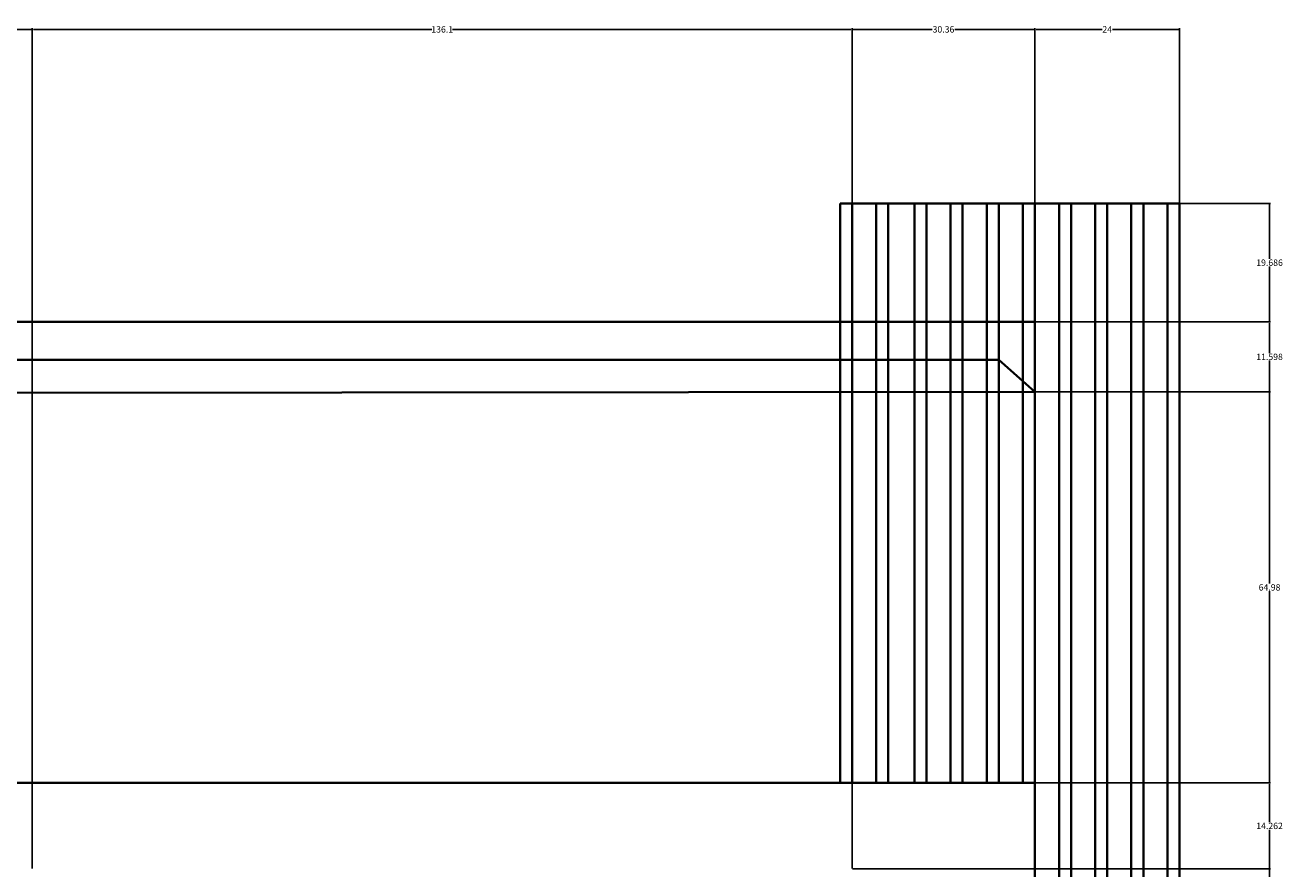
# Model space of a CAD drawing. Units: inches. Extents: x 35 to 365, y 67 to 380.
# Tile 5 of 5: x 156 to 365, y 240 to 380. Entities that reach past the tile are written whole.
import ezdxf

# ---------------------------------------------------------------- set-up
doc = ezdxf.new("R2010")
doc.units = ezdxf.units.IN
doc.header["$MEASUREMENT"] = 0
doc.layers.add('A-ANNO-DIMS', color=2, linetype='Continuous', lineweight=18)
doc.layers.add('A-FURN', color=7, linetype='Continuous', lineweight=35)
doc.styles.get("Standard").update_dxf_attribs({"font": 'arial.ttf'})
doc.dimstyles.get("Standard").update_dxf_attribs({"dimtxt": 1.0625, "dimasz": 0.18, "dimexe": 0.18, "dimexo": 0.0625, "dimgap": 0.09, "dimtad": 0, "dimtih": 1, "dimtoh": 1, "dimdec": 4, "dimzin": 0, "dimdsep": 46, "dimlunit": 4, "dimtxsty": 'Standard', "dimcen": 0.09, "dimadec": 0, "dimazin": 0, "dimtfac": 1, "dimtdec": 4, "dimtofl": 0, "dimtmove": 0, "dimatfit": 3, "dimfxl": 1, "dimtolj": 1, "dimtzin": 0, "dimarcsym": 0})

# ---------------------------------------------------------------- blocks, each defined once
blk = doc.blocks.new('*D12')
at = {"layer": 'A-ANNO-DIMS', "color": 0, "lineweight": -2, "transparency": 16777216}
for p, q in [((115.27, 351.36), (115.27, 379.42)), ((115.45, 379.24), (134.33, 379.24)), ((157.01, 379.24), (138.13, 379.24)), ((157.19, 239.87), (157.19, 379.42))]:
    blk.add_line(p, q, dxfattribs=at)
at = {"layer": 'A-ANNO-DIMS', "color": 0, "transparency": 16777216}
for points in [[(115.45, 379.27), (115.45, 379.21), (115.27, 379.24)], [(157.01, 379.27), (157.01, 379.21), (157.19, 379.24)]]:
    blk.add_solid(points, dxfattribs=at)
at = {"layer": 'Defpoints', "color": 0, "transparency": 16777216}
for p in [(157.19, 379.24), (115.27, 351.3), (157.19, 239.81)]:
    blk.add_point(p, dxfattribs=at)
at = {"layer": 'A-ANNO-DIMS', "color": 0, "transparency": 16777216, "insert": (136.23, 379.24), "char_height": 1.062, "attachment_point": 5}
blk.add_mtext('\\A1;41.92', dxfattribs=at)
blk = doc.blocks.new('*D13')
at = {"layer": 'A-ANNO-DIMS', "color": 0, "lineweight": -2, "transparency": 16777216}
for p, q in [((157.19, 239.87), (157.19, 379.42)), ((157.37, 379.24), (223.52, 379.24)), ((293.12, 379.24), (226.98, 379.24)), ((293.3, 239.87), (293.3, 379.42))]:
    blk.add_line(p, q, dxfattribs=at)
at = {"layer": 'A-ANNO-DIMS', "color": 0, "transparency": 16777216}
for points in [[(157.37, 379.27), (157.37, 379.21), (157.19, 379.24)], [(293.12, 379.27), (293.12, 379.21), (293.3, 379.24)]]:
    blk.add_solid(points, dxfattribs=at)
at = {"layer": 'Defpoints', "color": 0, "transparency": 16777216}
for p in [(293.3, 379.24), (157.19, 239.81), (293.3, 239.81)]:
    blk.add_point(p, dxfattribs=at)
at = {"layer": 'A-ANNO-DIMS', "color": 0, "transparency": 16777216, "insert": (225.25, 379.24), "char_height": 1.062, "attachment_point": 5}
blk.add_mtext('\\A1;136.1', dxfattribs=at)
blk = doc.blocks.new('*D14')
at = {"layer": 'A-ANNO-DIMS', "color": 0, "lineweight": -2, "transparency": 16777216}
for p, q in [((293.3, 239.87), (293.3, 379.42)), ((293.48, 379.24), (306.6, 379.24)), ((323.49, 379.24), (310.37, 379.24)), ((323.67, 350.4), (323.67, 379.42))]:
    blk.add_line(p, q, dxfattribs=at)
at = {"layer": 'A-ANNO-DIMS', "color": 0, "transparency": 16777216}
for points in [[(293.48, 379.27), (293.48, 379.21), (293.3, 379.24)], [(323.49, 379.27), (323.49, 379.21), (323.67, 379.24)]]:
    blk.add_solid(points, dxfattribs=at)
at = {"layer": 'Defpoints', "color": 0, "transparency": 16777216}
for p in [(323.67, 379.24), (323.67, 350.34), (293.3, 239.81)]:
    blk.add_point(p, dxfattribs=at)
at = {"layer": 'A-ANNO-DIMS', "color": 0, "transparency": 16777216, "insert": (308.48, 379.24), "char_height": 1.062, "attachment_point": 5}
blk.add_mtext('\\A1;30.36', dxfattribs=at)
blk = doc.blocks.new('*D15')
at = {"layer": 'A-ANNO-DIMS', "color": 0, "lineweight": -2, "transparency": 16777216}
for p, q in [((323.67, 350.4), (323.67, 379.42)), ((323.85, 379.24), (334.81, 379.24)), ((347.49, 379.24), (336.52, 379.24)), ((347.67, 350.4), (347.67, 379.42))]:
    blk.add_line(p, q, dxfattribs=at)
at = {"layer": 'A-ANNO-DIMS', "color": 0, "transparency": 16777216}
for points in [[(323.85, 379.27), (323.85, 379.21), (323.67, 379.24)], [(347.49, 379.27), (347.49, 379.21), (347.67, 379.24)]]:
    blk.add_solid(points, dxfattribs=at)
at = {"layer": 'Defpoints', "color": 0, "transparency": 16777216}
for p in [(347.67, 379.24), (323.67, 350.34), (347.67, 350.34)]:
    blk.add_point(p, dxfattribs=at)
at = {"layer": 'A-ANNO-DIMS', "color": 0, "transparency": 16777216, "insert": (335.67, 379.24), "char_height": 1.062, "attachment_point": 5}
blk.add_mtext('\\A1;24', dxfattribs=at)
blk = doc.blocks.new('*D26')
at = {"layer": 'A-ANNO-DIMS', "color": 0, "lineweight": -2, "transparency": 16777216}
for p, q in [((293.37, 239.81), (362.8, 239.81)), ((362.62, 239.63), (362.62, 203.07)), ((362.62, 165.26), (362.62, 201.82)), ((293.37, 165.08), (362.8, 165.08))]:
    blk.add_line(p, q, dxfattribs=at)
at = {"layer": 'A-ANNO-DIMS', "color": 0, "transparency": 16777216}
for points in [[(362.59, 239.63), (362.65, 239.63), (362.62, 239.81)], [(362.59, 165.26), (362.65, 165.26), (362.62, 165.08)]]:
    blk.add_solid(points, dxfattribs=at)
at = {"layer": 'Defpoints', "color": 0, "transparency": 16777216}
for p in [(293.3, 239.81), (362.62, 239.81), (293.3, 165.08)]:
    blk.add_point(p, dxfattribs=at)
at = {"layer": 'A-ANNO-DIMS', "color": 0, "transparency": 16777216, "insert": (362.62, 202.45), "char_height": 1.062, "attachment_point": 5}
blk.add_mtext('\\A1;74.72', dxfattribs=at)
blk = doc.blocks.new('*D27')
at = {"layer": 'A-ANNO-DIMS', "color": 0, "lineweight": -2, "transparency": 16777216}
for p, q in [((323.73, 254.07), (362.8, 254.07)), ((362.62, 253.89), (362.62, 247.57)), ((362.62, 239.99), (362.62, 246.31)), ((293.37, 239.81), (362.8, 239.81))]:
    blk.add_line(p, q, dxfattribs=at)
at = {"layer": 'A-ANNO-DIMS', "color": 0, "transparency": 16777216}
for points in [[(362.59, 253.89), (362.65, 253.89), (362.62, 254.07)], [(362.59, 239.99), (362.65, 239.99), (362.62, 239.81)]]:
    blk.add_solid(points, dxfattribs=at)
at = {"layer": 'Defpoints', "color": 0, "transparency": 16777216}
for p in [(323.67, 254.07), (362.62, 254.07), (293.3, 239.81)]:
    blk.add_point(p, dxfattribs=at)
at = {"layer": 'A-ANNO-DIMS', "color": 0, "transparency": 16777216, "insert": (362.62, 246.94), "char_height": 1.062, "attachment_point": 5}
blk.add_mtext('\\A1;14.262', dxfattribs=at)
blk = doc.blocks.new('*D28')
at = {"layer": 'A-ANNO-DIMS', "color": 0, "lineweight": -2, "transparency": 16777216}
for p, q in [((323.73, 319.05), (362.8, 319.05)), ((362.62, 318.87), (362.62, 287.19)), ((362.62, 254.25), (362.62, 285.93)), ((323.73, 254.07), (362.8, 254.07))]:
    blk.add_line(p, q, dxfattribs=at)
at = {"layer": 'A-ANNO-DIMS', "color": 0, "transparency": 16777216}
for points in [[(362.59, 318.87), (362.65, 318.87), (362.62, 319.05)], [(362.59, 254.25), (362.65, 254.25), (362.62, 254.07)]]:
    blk.add_solid(points, dxfattribs=at)
at = {"layer": 'Defpoints', "color": 0, "transparency": 16777216}
for p in [(323.67, 319.05), (362.62, 319.05), (323.67, 254.07)]:
    blk.add_point(p, dxfattribs=at)
at = {"layer": 'A-ANNO-DIMS', "color": 0, "transparency": 16777216, "insert": (362.62, 286.56), "char_height": 1.062, "attachment_point": 5}
blk.add_mtext('\\A1;64.98', dxfattribs=at)
blk = doc.blocks.new('*D29')
at = {"layer": 'A-ANNO-DIMS', "color": 0, "lineweight": -2, "transparency": 16777216}
for p, q in [((323.73, 330.65), (362.8, 330.65)), ((362.62, 330.47), (362.62, 325.48)), ((362.62, 319.23), (362.62, 324.22)), ((323.73, 319.05), (362.8, 319.05))]:
    blk.add_line(p, q, dxfattribs=at)
at = {"layer": 'A-ANNO-DIMS', "color": 0, "transparency": 16777216}
for points in [[(362.59, 330.47), (362.65, 330.47), (362.62, 330.65)], [(362.59, 319.23), (362.65, 319.23), (362.62, 319.05)]]:
    blk.add_solid(points, dxfattribs=at)
at = {"layer": 'Defpoints', "color": 0, "transparency": 16777216}
for p in [(323.67, 330.65), (362.62, 330.65), (323.67, 319.05)]:
    blk.add_point(p, dxfattribs=at)
at = {"layer": 'A-ANNO-DIMS', "color": 0, "transparency": 16777216, "insert": (362.62, 324.85), "char_height": 1.062, "attachment_point": 5}
blk.add_mtext('\\A1;11.598', dxfattribs=at)
blk = doc.blocks.new('*D30')
at = {"layer": 'A-ANNO-DIMS', "color": 0, "lineweight": -2, "transparency": 16777216}
for p, q in [((347.73, 350.34), (362.8, 350.34)), ((362.62, 350.16), (362.62, 341.13)), ((362.62, 330.83), (362.62, 339.86)), ((323.73, 330.65), (362.8, 330.65))]:
    blk.add_line(p, q, dxfattribs=at)
at = {"layer": 'A-ANNO-DIMS', "color": 0, "transparency": 16777216}
for points in [[(362.59, 350.16), (362.65, 350.16), (362.62, 350.34)], [(362.59, 330.83), (362.65, 330.83), (362.62, 330.65)]]:
    blk.add_solid(points, dxfattribs=at)
at = {"layer": 'Defpoints', "color": 0, "transparency": 16777216}
for p in [(347.67, 350.34), (362.62, 350.34), (323.67, 330.65)]:
    blk.add_point(p, dxfattribs=at)
at = {"layer": 'A-ANNO-DIMS', "color": 0, "transparency": 16777216, "insert": (362.62, 340.49), "char_height": 1.062, "attachment_point": 5}
blk.add_mtext('\\A1;19.686', dxfattribs=at)

msp = doc.modelspace()

# ---------------------------------------------------------------- linework, layer by layer
at = {"layer": 'A-FURN'}
for p, q in [((291.3029, 293.4266), (291.3029, 350.3365)), ((291.3029, 350.3365), (347.6655, 350.3365)), ((293.3029, 293.4266), (293.3029, 350.3365)), ((297.3029, 293.4266), (297.3029, 350.3365)), ((299.3029, 293.4266), (299.3029, 350.3365)), ((303.6655, 293.4266), (303.6655, 350.3365)), ((305.6655, 293.4266), (305.6655, 350.3365)), ((309.6655, 293.4266), (309.6655, 350.3365)), ((311.6655, 293.4266), (311.6655, 350.3365)), ((315.6655, 293.4266), (315.6655, 350.3365)), ((317.6655, 293.4266), (317.6655, 350.3365)), ((321.6655, 293.4266), (321.6655, 350.3365)), ((323.6655, 293.4266), (323.6655, 350.3365)), ((327.6655, 293.4266), (327.6655, 350.3365)), ((329.6655, 293.4266), (329.6655, 350.3365)), ((333.6655, 293.4266), (333.6655, 350.3365)), ((335.6655, 293.4266), (335.6655, 350.3365)), ((339.6655, 293.4266), (339.6655, 350.3365)), ((341.6655, 293.4266), (341.6655, 350.3365)), ((345.6655, 293.5027), (345.6655, 350.3365)), ((347.6655, 293.5027), (347.6655, 350.3365)), ((115.383, 330.6506), (323.6655, 330.6506)), ((323.6655, 330.6506), (323.6655, 319.0524)), ((119.5786, 324.3612), (317.6655, 324.3612)), ((317.6655, 324.3612), (323.6655, 319.0524)), ((323.6655, 319.0524), (115.383, 318.8192)), ((291.3029, 254.0695), (291.3029, 293.4266)), ((293.3029, 254.0695), (293.3029, 293.4266)), ((297.3029, 254.0695), (297.3029, 293.4266)), ((299.3029, 254.0695), (299.3029, 293.4266)), ((303.6655, 254.0695), (303.6655, 293.4266)), ((305.6655, 254.0695), (305.6655, 293.4266)), ((309.6655, 254.0695), (309.6655, 293.4266)), ((311.6655, 254.0695), (311.6655, 293.4266)), ((315.6655, 254.0695), (315.6655, 293.4266)), ((317.6655, 254.0695), (317.6655, 293.4266)), ((321.6655, 254.0695), (321.6655, 293.4266)), ((323.6655, 82.9768), (323.6655, 293.4266)), ((327.6655, 82.9768), (327.6655, 293.4266)), ((329.6655, 82.9768), (329.6655, 293.4266)), ((333.6655, 82.9768), (333.6655, 293.4266)), ((335.6655, 82.9768), (335.6655, 293.4266)), ((339.6655, 82.9768), (339.6655, 293.4266)), ((341.6655, 82.9768), (341.6655, 293.4266)), ((345.6655, 83.0529), (345.6655, 293.5027)), ((347.6655, 83.0529), (347.6655, 293.5027))]:
    msp.add_line(p, q, dxfattribs=at)
msp.add_lwpolyline([(115.383, 254.0695), (323.6655, 254.0695), (323.6655, 151.0198), (115.383, 151.0198)], close=True, dxfattribs=at)

# ---------------------------------------------------------------- dimensions: what is measured, and where the dimension line sits
at = {"layer": 'A-ANNO-DIMS'}
for base, p1, p2, override, picture, middle in [((157.1904, 379.2444), (115.273, 351.3011), (157.1904, 239.8076), {"dimdec": 2, "dimlfac": 1, "dimrnd": 0, "dimzin": 0, "dimdsep": 46, "dimlunit": 2}, '*D12', (136.2317, 379.2444)), ((293.3029, 379.2444), (157.1904, 239.8076), (293.3029, 239.8076), {"dimdec": 1, "dimlfac": 1, "dimrnd": 0, "dimzin": 0, "dimdsep": 46, "dimlunit": 2}, '*D13', (225.2467, 379.2444)), ((323.6655, 379.2444), (293.3029, 239.8076), (323.6655, 350.3365), {"dimdec": 2, "dimlfac": 1, "dimrnd": 0, "dimzin": 0, "dimdsep": 46, "dimlunit": 2}, '*D14', (308.4842, 379.2444)), ((347.6655, 379.2444), (323.6655, 350.3365), (347.6655, 350.3365), {"dimdec": 0, "dimlfac": 1, "dimrnd": 0, "dimzin": 0, "dimdsep": 46, "dimlunit": 2}, '*D15', (335.6655, 379.2444))]:
    dim = msp.add_linear_dim(base=base, p1=p1, p2=p2, dimstyle='Standard', override=override, dxfattribs=at)
    dim.commit()
    dim.dimension.update_dxf_attribs({"geometry": picture, "text_midpoint": middle})
for base, p1, p2, override, picture, middle in [((362.6155, 350.3365), (323.6655, 330.6506), (347.6655, 350.3365), {"dimdec": 3, "dimlfac": 1, "dimrnd": 0, "dimzin": 0, "dimdsep": 46, "dimlunit": 2}, '*D30', (362.6155, 340.4935)), ((362.6155, 330.6506), (323.6655, 319.0524), (323.6655, 330.6506), {"dimdec": 3, "dimlfac": 1, "dimrnd": 0, "dimzin": 0, "dimdsep": 46, "dimlunit": 2}, '*D29', (362.6155, 324.8515)), ((362.6155, 319.0524), (323.6655, 254.0695), (323.6655, 319.0524), {"dimdec": 2, "dimlfac": 1, "dimrnd": 0, "dimzin": 0, "dimdsep": 46, "dimlunit": 2}, '*D28', (362.6155, 286.561)), ((362.6155, 254.0695), (293.3029, 239.8076), (323.6655, 254.0695), {"dimdec": 3, "dimlfac": 1, "dimrnd": 0, "dimzin": 0, "dimdsep": 46, "dimlunit": 2}, '*D27', (362.6155, 246.9386)), ((362.6155, 239.8076), (293.3029, 165.0829), (293.3029, 239.8076), {"dimdec": 2, "dimlfac": 1, "dimrnd": 0, "dimzin": 0, "dimdsep": 46, "dimlunit": 2}, '*D26', (362.6155, 202.4453))]:
    dim = msp.add_linear_dim(base=base, p1=p1, p2=p2, angle=90, dimstyle='Standard', override=override, dxfattribs=at)
    dim.commit()
    dim.dimension.update_dxf_attribs({"geometry": picture, "text_midpoint": middle})

doc.saveas('drawing.dxf')
